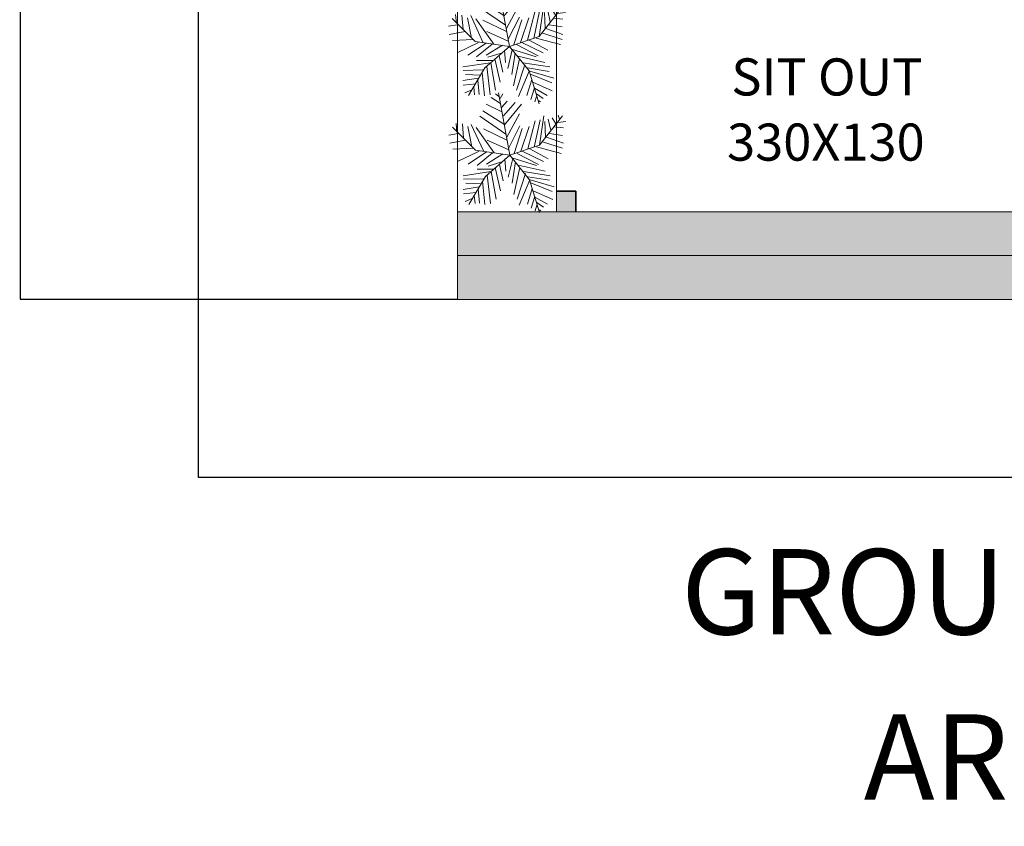
# Model space of a CAD drawing. Units: inches. Extents: x 192 to 1361, y -1362 to 367.
# Tile 1 of 23: x 192 to 649, y -1362 to -987. Entities that reach past the tile are written whole.
import ezdxf

# ---------------------------------------------------------------- set-up
doc = ezdxf.new("R2010")
doc.units = ezdxf.units.IN
doc.header["$MEASUREMENT"] = 0
for name, color, linetype, lineweight in [('A-ANNO-DIMS', 2, 'Continuous', 18), ('A-ANNO-TITL', 7, 'Continuous', 35), ('A-AREA-IDEN', 7, 'Continuous', 18), ('A-FLOR', 8, 'Continuous', 18), ('A-FLOR-STRS', 7, 'Continuous', 18), ('A-WALL-PATT', 250, 'Continuous', 13), ('lawn', 96, 'Continuous', 13), ('walls', 7, 'Continuous', 35)]:
    doc.layers.add(name, color=color, linetype=linetype, lineweight=lineweight)
doc.layers.add('A-FLOR-STRS-PATT', color=252, linetype='Continuous', lineweight=13, true_color=0x939598)
doc.styles.get("Standard").update_dxf_attribs({"font": 'arial.ttf'})
doc.dimstyles.get("Standard").update_dxf_attribs({"dimtxt": 0.18, "dimasz": 0.18, "dimexe": 0.18, "dimexo": 0.0625, "dimgap": 0.09, "dimtad": 0, "dimtih": 1, "dimtoh": 1, "dimzin": 0, "dimdsep": 46, "dimlunit": 3, "dimtxsty": 'Standard', "dimcen": 0.09, "dimadec": 0, "dimazin": 0, "dimtfac": 1, "dimtofl": 0, "dimtmove": 0, "dimatfit": 3, "dimfxl": 1, "dimtolj": 1, "dimtzin": 0, "dimarcsym": 0})

# ---------------------------------------------------------------- blocks, each defined once
blk = doc.blocks.new('*U4')
for p, q in [((-10.186, 53.64), (-13.084, 55.962)), ((0, 0), (-10.5, 57)), ((-9.099, 51.782), (-6.563, 55.962)), ((-7.288, 39.707), (-21.778, 46.673)), ((-8.737, 47.138), (-17.069, 52.711)), ((-7.65, 43.423), (-2.578, 49.46)), ((-5.839, 35.992), (4.667, 48.067)), ((-5.114, 27.632), (10.463, 46.673)), ((-5.114, 28.097), (-24.676, 40.636)), ((-2.941, 16.486), (8.652, 37.85)), ((44.153, 36.456), (45.239, 32.741)), ((-48.585, 21.131), (-49.309, 29.026)), ((-43.513, 28.561), (-42.427, 15.558)), ((-35.544, 28.097), (-24.314, 3.947)), ((-3.665, 19.273), (-27.574, 35.527)), ((16.259, 5.805), (23.142, 31.348)), ((22.055, 7.198), (27.489, 32.277)), ((27, 9), (48, 36)), ((27.127, 9.056), (31.112, 35.992)), ((31.836, 30.883), (32.561, 16.486)), ((35.096, 32.741), (37.27, 22.524)), ((38.719, 34.134), (41.979, 28.561)), ((43.791, 29.954), (51.036, 30.883)), ((-47.498, 19.737), (-55.83, 18.344)), ((-31.5, 4.5), (-52.5, 25.5)), ((-38.442, 26.239), (-34.819, 7.663)), ((-14.533, 2.09), (-30.834, 25.31)), ((-24.314, 23.917), (-2.941, 13.7)), ((-1.129, 6.734), (9.014, 26.704)), ((3.942, 1.625), (11.187, 24.381)), ((10.101, 3.483), (17.708, 26.239)), ((36.183, 19.737), (48.137, 17.88)), ((40.53, 25.775), (48.862, 24.846)), ((-40.615, 13.7), (-55.105, 10.913)), ((-20.691, 13.7), (-1.129, 4.876)), ((29.662, 12.307), (48.137, 6.269)), ((33.285, 16.486), (48.862, 10.913)), ((-33.37, 6.269), (-52.207, 5.34)), ((-28.299, 3.483), (-47.86, -5.805)), ((-21.416, 3.018), (-38.079, -8.128)), ((0, 0), (-31.5, 4.5)), ((-15.982, 2.09), (-30.11, -9.521)), ((0, 0), (-22.5, -19.5)), ((-6.563, 1.161), (-21.416, -8.128)), ((0, 0), (27, 9)), ((0, 0), (18, -22.5)), ((6.478, 1.625), (26.04, -8.592)), ((11.187, 3.483), (30.749, -5.805)), ((18.07, 5.805), (35.096, -3.483)), ((24.229, 7.663), (46.688, 1.625)), ((-6.563, -5.805), (-19.967, -9.985)), ((-9.461, -8.592), (-6.201, -23.453)), ((-4.752, -3.483), (-3.665, -14.629)), ((2.493, -3.019), (-1.491, -20.202)), ((1.769, -2.555), (24.229, -9.521)), ((5.029, -6.27), (2.131, -25.775)), ((-17.431, -15.094), (-42.789, -18.809)), ((-15.257, -12.772), (-30.11, -12.772)), ((-17.069, -15.094), (-12.721, -40.172)), ((-13.446, -11.378), (-8.737, -32.741)), ((9.014, -11.378), (3.58, -35.992)), ((14.085, -16.951), (6.478, -40.172)), ((7.565, -9.056), (32.198, -14.629)), ((12.274, -15.094), (36.907, -18.809)), ((-24.314, -21.596), (-42.427, -22.06)), ((-26.849, -26.24), (-40.253, -25.775)), ((-22.5, -19.5), (-37.5, -45)), ((-25.038, -23.918), (-22.865, -45.281)), ((-20.691, -18.345), (-17.793, -44.352)), ((18.07, -22.524), (8.289, -45.745)), ((16.259, -19.738), (36.183, -22.989)), ((18, -22.5), (27, -52.5)), ((18.433, -22.524), (40.53, -29.026)), ((19.157, -25.311), (38.719, -33.206)), ((-28.299, -29.026), (-42.789, -31.348)), ((-30.834, -34.135), (-42.427, -35.528)), ((-29.023, -30.884), (-27.936, -43.887)), ((20.244, -30.419), (15.897, -44.816)), ((21.331, -32.741), (39.081, -40.636)), ((-34.457, -39.708), (-40.978, -42.494)), ((-32.646, -36.921), (-31.921, -44.352)), ((22.78, -37.85), (19.519, -48.532)), ((22.78, -38.314), (34.372, -44.816)), ((24.591, -43.423), (30.749, -47.603)), ((24.591, -45.745), (23.142, -50.854)), ((26.764, -49.925), (28.213, -50.854))]:
    blk.add_line(p, q)
blk = doc.blocks.new('*D47')
at = {"layer": 'A-ANNO-DIMS', "color": 0, "lineweight": -2, "transparency": 16777216}
for p, q in [((1273.57, -782.95), (1273.57, -1200.05)), ((274.89, -914.5), (274.89, -1200.05)), ((275.07, -1199.87), (773.84, -1199.87)), ((1273.39, -1199.87), (774.62, -1199.87))]:
    blk.add_line(p, q, dxfattribs=at)
at = {"layer": 'A-ANNO-DIMS', "color": 0, "transparency": 16777216}
for points in [[(275.07, -1199.84), (275.07, -1199.9), (274.89, -1199.87)], [(1273.39, -1199.84), (1273.39, -1199.9), (1273.57, -1199.87)]]:
    blk.add_solid(points, dxfattribs=at)
at = {"layer": 'Defpoints', "color": 0, "transparency": 16777216}
for p in [(1273.57, -782.89), (274.89, -914.44), (1273.57, -1199.87)]:
    blk.add_point(p, dxfattribs=at)
at = {"layer": 'A-ANNO-DIMS', "color": 0, "transparency": 16777216, "insert": (774.23, -1199.87), "char_height": 0.18, "attachment_point": 5}
blk.add_mtext('\\A1;998.7', dxfattribs=at)
blk = doc.blocks.new('*D48')
at = {"layer": 'A-ANNO-DIMS', "color": 0, "lineweight": -2, "transparency": 16777216}
for p, q in [((325.63, 258.53), (192.16, 258.53)), ((192.34, 258.35), (192.34, -429.22)), ((192.34, -1117.14), (192.34, -429.58)), ((395.21, -1117.32), (192.16, -1117.32))]:
    blk.add_line(p, q, dxfattribs=at)
at = {"layer": 'A-ANNO-DIMS', "color": 0, "transparency": 16777216}
for points in [[(192.31, 258.35), (192.37, 258.35), (192.34, 258.53)], [(192.31, -1117.14), (192.37, -1117.14), (192.34, -1117.32)]]:
    blk.add_solid(points, dxfattribs=at)
at = {"layer": 'Defpoints', "color": 0, "transparency": 16777216}
for p in [(325.7, 258.53), (192.34, -1117.32), (395.28, -1117.32)]:
    blk.add_point(p, dxfattribs=at)
at = {"layer": 'A-ANNO-DIMS', "color": 0, "transparency": 16777216, "insert": (192.34, -429.4), "char_height": 0.18, "attachment_point": 5}
blk.add_mtext('\\A1;1375.9', dxfattribs=at)

msp = doc.modelspace()

# ---------------------------------------------------------------- hatches: boundary and pattern name
at = {"layer": 'A-FLOR-STRS-PATT'}
h = msp.add_hatch(color=256, dxfattribs=at)
h.dxf.hatch_style = 1
h.paths.add_polyline_path([(781.5537, -1096.9736), (395.2768, -1096.9736), (395.2768, -1117.3227), (781.5537, -1117.3227)])
h.paths.add_polyline_path([(781.5537, -1076.6246), (749.8458, -1076.6246), (441.307, -1076.6246), (395.2768, -1076.6246), (395.2768, -1096.9736), (781.5537, -1096.9736)])
at = {"layer": 'A-WALL-PATT'}
h = msp.add_hatch(color=256, dxfattribs=at)
h.dxf.hatch_style = 1
h.paths.add_polyline_path([(309.5452, 191.102), (300.5452, 191.102), (300.5452, -126.898), (309.5452, -126.898), (309.5452, -117.898)])
h.paths.add_polyline_path([(420.798, 191.102), (337.3229, 191.102), (337.3229, 182.102), (420.798, 182.102)])
h.paths.add_polyline_path([(518.5452, 182.102), (625.4022, 182.102), (625.4022, 191.102), (509.5452, 191.102), (509.5452, 114.3262), (518.5452, 114.3262)])
h.paths.add_polyline_path([(842.5452, 191.102), (763.4438, 191.102), (763.4438, 182.102), (833.5452, 182.102), (833.5452, 161.1615), (836.8088, 161.1615), (842.5452, 161.1615)])
h.paths.add_polyline_path([(842.5452, -16.5675), (833.5452, -16.5675), (833.5452, -60.4996), (784.8041, -60.4996), (784.8041, -354.6796), (793.8041, -354.6796), (793.8041, -69.4996), (1094.1252, -69.4996), (1094.1252, -60.4996), (842.5452, -60.4996)])
h.paths.add_polyline_path([(518.5452, 36.602), (509.5452, 36.602), (509.5452, -117.898), (420.2204, -117.898), (420.2204, -126.898), (518.5452, -126.898)])
h.paths.add_polyline_path([(474.8041, -377.0384), (465.8041, -377.0384), (465.8041, -381.5384), (465.8041, -450.898), (537.5717, -450.898), (537.5717, -441.898), (474.8041, -441.898)])
h.paths.add_polyline_path([(1162.8041, -380.6763), (1204.3001, -380.6763), (1204.3001, -375.6763), (1195.1471, -375.6763), (1153.8041, -375.6763), (1153.8041, -448.4996), (856.5691, -448.4996), (856.5691, -457.4996), (1162.8041, -457.4996)])
h.paths.add_polyline_path([(1162.8041, -525.128), (1153.8041, -525.128), (1153.8041, -597.4996), (1162.8041, -597.4996)], flags=17)
h.paths.add_polyline_path([(1162.8041, -60.4996), (1153.8041, -60.4996), (1153.8041, -69.4996), (1153.8041, -177.4733), (1205.8889, -177.4733), (1205.8889, -172.4733), (1162.8041, -172.4733)])
h.paths.add_polyline_path([(980.5799, -525.686), (971.5799, -525.686), (971.5799, -597.4996), (980.5799, -597.4996)], flags=17)
h.paths.add_polyline_path([(856.5691, -448.4996), (798.7542, -448.4996), (784.8041, -448.4996), (784.8041, -457.4996), (847.5691, -457.4996), (847.5691, -597.4996), (784.8041, -597.4996), (784.8041, -606.4996), (1273.5658, -606.4996), (1273.5658, -597.4996), (856.5691, -597.4996)])
h.paths.add_polyline_path([(1273.5658, -773.892), (1099.8366, -773.892), (1099.8366, -851.9362), (1108.8366, -851.9362), (1108.8366, -782.892), (1273.5658, -782.892)])
h.paths.add_polyline_path([(1108.8366, -982.9214), (1099.8366, -982.9214), (1099.8366, -1067.6246), (1037.7563, -1067.6246), (1037.7563, -1076.6246), (1108.8366, -1076.6246)])
h.paths.add_polyline_path([(835.078, -1067.6246), (758.8458, -1067.6246), (758.8458, -940.2324), (749.8458, -940.2324), (749.8458, -963.172), (749.8458, -970.4644), (749.8458, -1076.6246), (835.078, -1076.6246)])
h.paths.add_polyline_path([(450.307, -1066.9838), (441.307, -1066.9838), (441.307, -1076.6246), (450.307, -1076.6246)])
h.paths.add_polyline_path([(492.8925, -756.4415), (274.8925, -756.4415), (274.8925, -765.4415), (492.8925, -765.4415)])
h.paths.add_polyline_path([(283.8925, -835.2244), (274.8925, -835.2244), (274.8925, -914.4415), (492.8925, -914.4415), (492.8925, -839.9415), (483.8925, -839.9415), (483.8925, -905.4415), (283.8925, -905.4415)])
h.paths.add_polyline_path([(283.8925, -441.898), (283.8925, -375.4296), (281.6021, -375.4296), (281.6021, -399.4121), (274.8925, -399.4121), (274.8925, -441.898), (274.8925, -684.5089), (283.8925, -684.5089)])

# ---------------------------------------------------------------- linework, layer by layer
at = {"layer": 'A-FLOR'}
for p, q in [((395.2768, -1076.6246), (395.2768, -914.4415)), ((441.307, -1076.6246), (441.307, -969.5484)), ((749.8458, -1076.6246), (441.307, -1076.6246))]:
    msp.add_line(p, q, dxfattribs=at)
at = {"layer": 'A-FLOR-STRS'}
for p, q in [((441.307, -1076.6246), (395.2768, -1076.6246)), ((395.2768, -1076.6246), (395.2768, -1117.3227)), ((395.2768, -1096.9736), (781.5537, -1096.9736)), ((395.2768, -1117.3227), (781.5537, -1117.3227))]:
    msp.add_line(p, q, dxfattribs=at)
at = {"layer": 'walls'}
for p, q in [((450.307, -1066.9838), (441.307, -1066.9838)), ((450.307, -1076.6246), (450.307, -1066.9838))]:
    msp.add_line(p, q, dxfattribs=at)

# ---------------------------------------------------------------- block references
at = {"layer": 'lawn', "xscale": 0.5078671948952364, "yscale": 0.5078671948952364, "zscale": 0.5078671948952364}
for p in [(419.4939, -999.7959), (419.678, -1050.3074)]:
    msp.add_blockref('*U4', p, dxfattribs=at)

# ---------------------------------------------------------------- texts
at = {"layer": 'A-ANNO-TITL'}
for s, p in [('GROUND FLOOR PLAN', (499.1662, -1272.9554)), ('AREA - 1238 sqft', (584.0247, -1349.6751))]:
    msp.add_text(s, height=39.646878, dxfattribs=at).set_placement(p)
at = {"layer": 'A-AREA-IDEN'}
for s, p in [('SIT OUT', (522.4963, -1022.6083)), ('330X130', (520.5104, -1052.881))]:
    msp.add_text(s, height=17.23824, dxfattribs=at).set_placement(p)

# ---------------------------------------------------------------- dimensions: what is measured, and where the dimension line sits
at = {"layer": 'A-ANNO-DIMS'}
dim = msp.add_linear_dim(base=(192.3425, -1117.3227), p1=(325.6957, 258.5286), p2=(395.2768, -1117.3227), angle=90, dimstyle='Standard', override={"dimdec": 1, "dimlfac": 1, "dimrnd": 0, "dimzin": 0, "dimdsep": 46, "dimlunit": 2}, dxfattribs=at)
dim.commit()
dim.dimension.update_dxf_attribs({"geometry": '*D48', "text_midpoint": (192.3425, -429.3971)})
dim = msp.add_linear_dim(base=(1273.5658, -1199.8727), p1=(274.8925, -914.4415), p2=(1273.5658, -782.892), dimstyle='Standard', override={"dimdec": 1, "dimlfac": 1, "dimrnd": 0, "dimzin": 0, "dimdsep": 46, "dimlunit": 2}, dxfattribs=at)
dim.commit()
dim.dimension.update_dxf_attribs({"geometry": '*D47', "text_midpoint": (774.2292, -1199.8727)})

doc.saveas('drawing.dxf')
